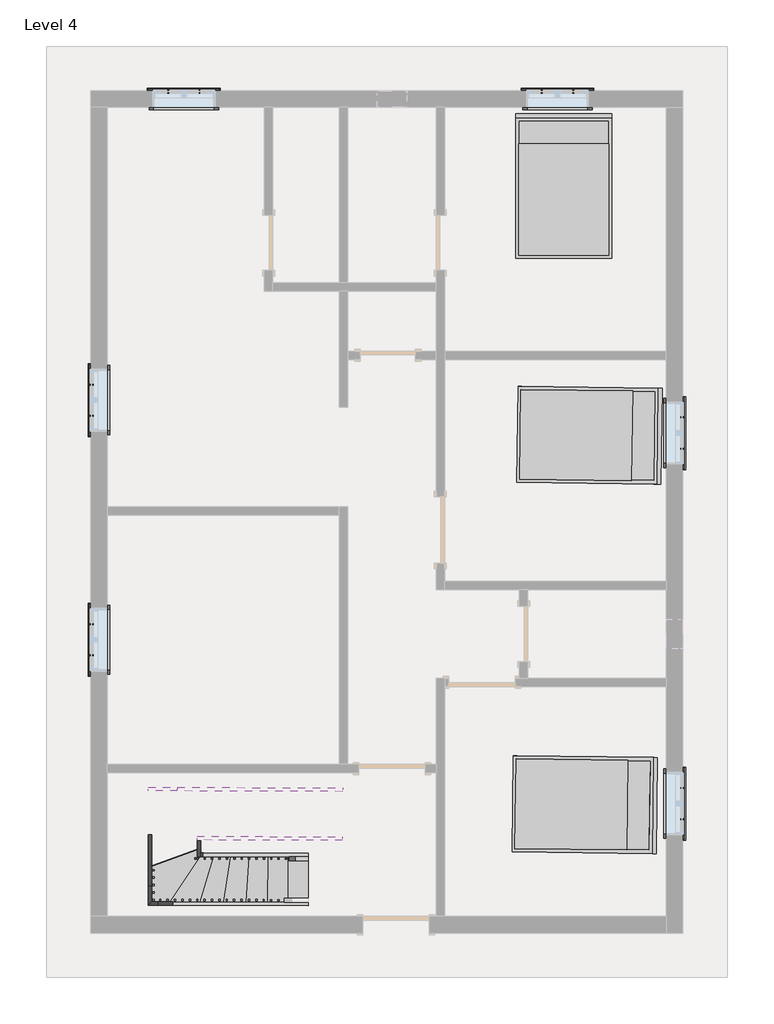
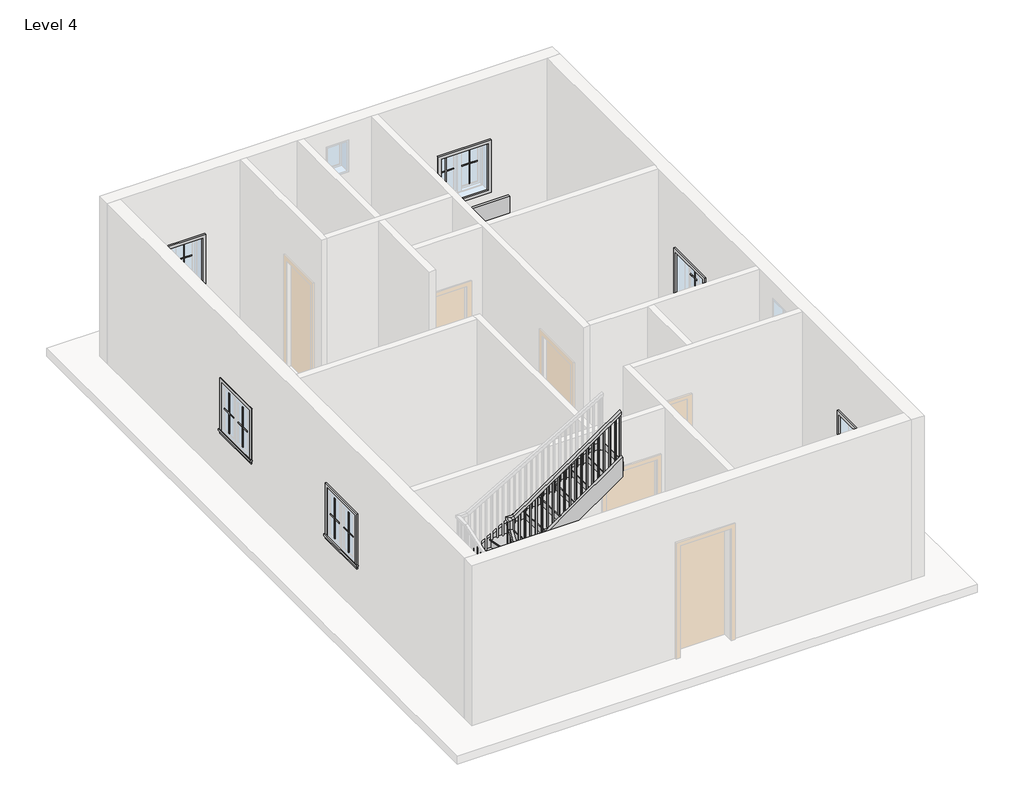
# One storey, part 3 of 3: 24 proxies, 9 members, 3 furniture elements, 1 railing, 1 stair flight.
"""IFC4 building model written with IfcOpenShell, lengths in millimetres."""

from ifc_helpers import new_model, si_unit, frame, origin, place, context, project, spatial, polyline, outline, extrude, faceted_brep, transform, mapped, element, save
from components import muntin_pattern_2x2_muntin_pattern_2x2_b3fe6957, muntin_pattern_2x2_muntin_pattern_2x2_3e0ecaf2, trim_window_exterior_flat_with_sill_41619996, trim_window_interior_flat_picture_frame_51c85655, bed_17739_bed_17739_15c61121, stair_flight_f5e35143

model = new_model("IFC4")

# Units and contexts
model_context = context("Model", 3, world=origin())
ifc_project = project(units=[si_unit("LENGTHUNIT", "METRE", prefix="MILLI")], contexts=[model_context])

# Site, building, storey
site = spatial("IfcSite", under=ifc_project)
building = spatial("IfcBuilding", under=site)
storey = spatial("IfcBuildingStorey", under=building, Name="Level 4", Elevation=6400.8)

# Proxies
placement = place(None, origin())
muntin_pattern_2x2_muntin_pattern_2x2_shape = muntin_pattern_2x2_muntin_pattern_2x2_b3fe6957(model_context)
element("IfcBuildingElementProxy", 1, Name="Muntin Pattern_2x2 : Muntin Pattern_2x2", ObjectType="Muntin Pattern_2x2 : Muntin Pattern_2x2", at=placement, inside=storey, context=model_context, shape_type="MappedRepresentation", body=[
    mapped(muntin_pattern_2x2_muntin_pattern_2x2_shape, transform((873.7257686, 6321.6571212, 7385.05), x_axis=(1.0, 0.0, 0.0), y_axis=(0.0, 1.0, 0.0), z_axis=(0.0, 0.0, 1.0))),
])
element("IfcBuildingElementProxy", 2, Name="Muntin Pattern_2x2 : Muntin Pattern_2x2", ObjectType="Muntin Pattern_2x2 : Muntin Pattern_2x2", at=placement, inside=storey, context=model_context, shape_type="MappedRepresentation", body=[
    mapped(muntin_pattern_2x2_muntin_pattern_2x2_shape, transform((2802.5382686, 1840.1446212, 7385.05), x_axis=(0.0, -1.0, 0.0), y_axis=(1.0, 0.0, 0.0), z_axis=(0.0, 0.0, 1.0))),
])
element("IfcBuildingElementProxy", 3, Name="Muntin Pattern_2x2 : Muntin Pattern_2x2", ObjectType="Muntin Pattern_2x2 : Muntin Pattern_2x2", at=placement, inside=storey, context=model_context, shape_type="MappedRepresentation", body=[
    mapped(muntin_pattern_2x2_muntin_pattern_2x2_shape, transform((2802.5382686, -3255.7303788, 7385.05), x_axis=(0.0, -1.0, 0.0), y_axis=(1.0, 0.0, 0.0), z_axis=(0.0, 0.0, 1.0))),
])
element("IfcBuildingElementProxy", 4, Name="Muntin Pattern_2x2 : Muntin Pattern_2x2", ObjectType="Muntin Pattern_2x2 : Muntin Pattern_2x2", at=placement, inside=storey, context=model_context, shape_type="MappedRepresentation", body=[
    mapped(muntin_pattern_2x2_muntin_pattern_2x2_shape, transform((-4263.4242314, 6321.6571212, 7385.05), x_axis=(1.0, 0.0, 0.0), y_axis=(0.0, 1.0, 0.0), z_axis=(0.0, 0.0, 1.0))),
])
element("IfcBuildingElementProxy", 5, Name="Muntin Pattern_2x2 : Muntin Pattern_2x2", ObjectType="Muntin Pattern_2x2 : Muntin Pattern_2x2", at=placement, inside=storey, context=model_context, shape_type="MappedRepresentation", body=[
    mapped(muntin_pattern_2x2_muntin_pattern_2x2_shape, transform((-5319.1117314, 1863.8332318, 7385.05), x_axis=(0.0, 1.0, 0.0), y_axis=(-1.0, 0.0, 0.0), z_axis=(0.0, 0.0, 1.0))),
])
element("IfcBuildingElementProxy", 6, Name="Muntin Pattern_2x2 : Muntin Pattern_2x2", ObjectType="Muntin Pattern_2x2 : Muntin Pattern_2x2", at=placement, inside=storey, context=model_context, shape_type="MappedRepresentation", body=[
    mapped(muntin_pattern_2x2_muntin_pattern_2x2_shape, transform((-5319.1117314, -1431.8167682, 7385.05), x_axis=(0.0, 1.0, 0.0), y_axis=(-1.0, 0.0, 0.0), z_axis=(0.0, 0.0, 1.0))),
])
muntin_pattern_2x2_muntin_pattern_2x2_2_shape = muntin_pattern_2x2_muntin_pattern_2x2_3e0ecaf2(model_context)
element("IfcBuildingElementProxy", 7, Name="Muntin Pattern_2x2 : Muntin Pattern_2x2", ObjectType="Muntin Pattern_2x2 : Muntin Pattern_2x2", at=placement, inside=storey, context=model_context, shape_type="MappedRepresentation", body=[
    mapped(muntin_pattern_2x2_muntin_pattern_2x2_2_shape, transform((1302.3507686, 6321.6571212, 7385.05), x_axis=(-1.0, 0.0, 0.0), y_axis=(0.0, -1.0, 0.0), z_axis=(0.0, 0.0, 1.0))),
])
element("IfcBuildingElementProxy", 8, Name="Muntin Pattern_2x2 : Muntin Pattern_2x2", ObjectType="Muntin Pattern_2x2 : Muntin Pattern_2x2", at=placement, inside=storey, context=model_context, shape_type="MappedRepresentation", body=[
    mapped(muntin_pattern_2x2_muntin_pattern_2x2_2_shape, transform((2802.5382686, 1411.5196212, 7385.05), x_axis=(0.0, 1.0, 0.0), y_axis=(-1.0, 0.0, 0.0), z_axis=(0.0, 0.0, 1.0))),
])
element("IfcBuildingElementProxy", 9, Name="Muntin Pattern_2x2 : Muntin Pattern_2x2", ObjectType="Muntin Pattern_2x2 : Muntin Pattern_2x2", at=placement, inside=storey, context=model_context, shape_type="MappedRepresentation", body=[
    mapped(muntin_pattern_2x2_muntin_pattern_2x2_2_shape, transform((2802.5382686, -3684.3553788, 7385.05), x_axis=(0.0, 1.0, 0.0), y_axis=(-1.0, 0.0, 0.0), z_axis=(0.0, 0.0, 1.0))),
])
element("IfcBuildingElementProxy", 10, Name="Muntin Pattern_2x2 : Muntin Pattern_2x2", ObjectType="Muntin Pattern_2x2 : Muntin Pattern_2x2", at=placement, inside=storey, context=model_context, shape_type="MappedRepresentation", body=[
    mapped(muntin_pattern_2x2_muntin_pattern_2x2_2_shape, transform((-3834.7992314, 6321.6571212, 7385.05), x_axis=(-1.0, 0.0, 0.0), y_axis=(0.0, -1.0, 0.0), z_axis=(0.0, 0.0, 1.0))),
])
element("IfcBuildingElementProxy", 11, Name="Muntin Pattern_2x2 : Muntin Pattern_2x2", ObjectType="Muntin Pattern_2x2 : Muntin Pattern_2x2", at=placement, inside=storey, context=model_context, shape_type="MappedRepresentation", body=[
    mapped(muntin_pattern_2x2_muntin_pattern_2x2_2_shape, transform((-5319.1117314, 2292.4582318, 7385.05), x_axis=(0.0, -1.0, 0.0), y_axis=(1.0, 0.0, 0.0), z_axis=(0.0, 0.0, 1.0))),
])
element("IfcBuildingElementProxy", 12, Name="Muntin Pattern_2x2 : Muntin Pattern_2x2", ObjectType="Muntin Pattern_2x2 : Muntin Pattern_2x2", at=placement, inside=storey, context=model_context, shape_type="MappedRepresentation", body=[
    mapped(muntin_pattern_2x2_muntin_pattern_2x2_2_shape, transform((-5319.1117314, -1003.1917682, 7385.05), x_axis=(0.0, -1.0, 0.0), y_axis=(1.0, 0.0, 0.0), z_axis=(0.0, 0.0, 1.0))),
])
trim_window_exterior_flat_with_sill_shape = trim_window_exterior_flat_with_sill_41619996(model_context)
element("IfcBuildingElementProxy", 13, Name="Trim-Window-Exterior-Flat : with Sill", ObjectType="Trim-Window-Exterior-Flat : with Sill", at=placement, inside=storey, context=model_context, shape_type="MappedRepresentation", body=[
    mapped(trim_window_exterior_flat_with_sill_shape, transform((1088.0382686, 6331.1821212, 8229.6), x_axis=(-1.0, 0.0, 0.0), y_axis=(0.0, 0.0, 1.0), z_axis=(0.0, 1.0, 0.0))),
])
element("IfcBuildingElementProxy", 14, Name="Trim-Window-Exterior-Flat : with Sill", ObjectType="Trim-Window-Exterior-Flat : with Sill", at=placement, inside=storey, context=model_context, shape_type="MappedRepresentation", body=[
    mapped(trim_window_exterior_flat_with_sill_shape, transform((2812.0632686, 1625.8321212, 8229.6), x_axis=(0.0, 1.0, 0.0), y_axis=(0.0, 0.0, 1.0), z_axis=(1.0, 0.0, 0.0))),
])
element("IfcBuildingElementProxy", 15, Name="Trim-Window-Exterior-Flat : with Sill", ObjectType="Trim-Window-Exterior-Flat : with Sill", at=placement, inside=storey, context=model_context, shape_type="MappedRepresentation", body=[
    mapped(trim_window_exterior_flat_with_sill_shape, transform((2812.0632686, -3470.0428788, 8229.6), x_axis=(0.0, 1.0, 0.0), y_axis=(0.0, 0.0, 1.0), z_axis=(1.0, 0.0, 0.0))),
])
element("IfcBuildingElementProxy", 16, Name="Trim-Window-Exterior-Flat : with Sill", ObjectType="Trim-Window-Exterior-Flat : with Sill", at=placement, inside=storey, context=model_context, shape_type="MappedRepresentation", body=[
    mapped(trim_window_exterior_flat_with_sill_shape, transform((-4049.1117314, 6331.1821212, 8229.6), x_axis=(-1.0, 0.0, 0.0), y_axis=(0.0, 0.0, 1.0), z_axis=(0.0, 1.0, 0.0))),
])
element("IfcBuildingElementProxy", 17, Name="Trim-Window-Exterior-Flat : with Sill", ObjectType="Trim-Window-Exterior-Flat : with Sill", at=placement, inside=storey, context=model_context, shape_type="MappedRepresentation", body=[
    mapped(trim_window_exterior_flat_with_sill_shape, transform((-5328.6367314, 2078.1457318, 8229.6), x_axis=(0.0, -1.0, 0.0), y_axis=(0.0, 0.0, 1.0), z_axis=(-1.0, 0.0, 0.0))),
])
element("IfcBuildingElementProxy", 18, Name="Trim-Window-Exterior-Flat : with Sill", ObjectType="Trim-Window-Exterior-Flat : with Sill", at=placement, inside=storey, context=model_context, shape_type="MappedRepresentation", body=[
    mapped(trim_window_exterior_flat_with_sill_shape, transform((-5328.6367314, -1217.5042682, 8229.6), x_axis=(0.0, -1.0, 0.0), y_axis=(0.0, 0.0, 1.0), z_axis=(-1.0, 0.0, 0.0))),
])
trim_window_interior_flat_picture_frame_shape = trim_window_interior_flat_picture_frame_51c85655(model_context)
element("IfcBuildingElementProxy", 19, Name="Trim-Window-Interior-Flat : Picture Frame", ObjectType="Trim-Window-Interior-Flat : Picture Frame", at=placement, inside=storey, context=model_context, shape_type="MappedRepresentation", body=[
    mapped(trim_window_interior_flat_picture_frame_shape, transform((1088.0382686, 6102.5821212, 8229.6), x_axis=(1.0, 0.0, 0.0), y_axis=(0.0, 0.0, 1.0), z_axis=(0.0, -1.0, 0.0))),
])
element("IfcBuildingElementProxy", 20, Name="Trim-Window-Interior-Flat : Picture Frame", ObjectType="Trim-Window-Interior-Flat : Picture Frame", at=placement, inside=storey, context=model_context, shape_type="MappedRepresentation", body=[
    mapped(trim_window_interior_flat_picture_frame_shape, transform((2583.4632686, 1625.8321212, 8229.6), x_axis=(0.0, -1.0, 0.0), y_axis=(0.0, 0.0, 1.0), z_axis=(-1.0, 0.0, 0.0))),
])
element("IfcBuildingElementProxy", 21, Name="Trim-Window-Interior-Flat : Picture Frame", ObjectType="Trim-Window-Interior-Flat : Picture Frame", at=placement, inside=storey, context=model_context, shape_type="MappedRepresentation", body=[
    mapped(trim_window_interior_flat_picture_frame_shape, transform((2583.4632686, -3470.0428788, 8229.6), x_axis=(0.0, -1.0, 0.0), y_axis=(0.0, 0.0, 1.0), z_axis=(-1.0, 0.0, 0.0))),
])
element("IfcBuildingElementProxy", 22, Name="Trim-Window-Interior-Flat : Picture Frame", ObjectType="Trim-Window-Interior-Flat : Picture Frame", at=placement, inside=storey, context=model_context, shape_type="MappedRepresentation", body=[
    mapped(trim_window_interior_flat_picture_frame_shape, transform((-4049.1117314, 6102.5821212, 8229.6), x_axis=(1.0, 0.0, 0.0), y_axis=(0.0, 0.0, 1.0), z_axis=(0.0, -1.0, 0.0))),
])
element("IfcBuildingElementProxy", 23, Name="Trim-Window-Interior-Flat : Picture Frame", ObjectType="Trim-Window-Interior-Flat : Picture Frame", at=placement, inside=storey, context=model_context, shape_type="MappedRepresentation", body=[
    mapped(trim_window_interior_flat_picture_frame_shape, transform((-5100.0367314, 2078.1457318, 8229.6), x_axis=(0.0, 1.0, 0.0), y_axis=(0.0, 0.0, 1.0), z_axis=(1.0, 0.0, 0.0))),
])
element("IfcBuildingElementProxy", 24, Name="Trim-Window-Interior-Flat : Picture Frame", ObjectType="Trim-Window-Interior-Flat : Picture Frame", at=placement, inside=storey, context=model_context, shape_type="MappedRepresentation", body=[
    mapped(trim_window_interior_flat_picture_frame_shape, transform((-5100.0367314, -1217.5042682, 8229.6), x_axis=(0.0, 1.0, 0.0), y_axis=(0.0, 0.0, 1.0), z_axis=(1.0, 0.0, 0.0))),
])

# Furniture
bed_17739_bed_17739_shape = bed_17739_bed_17739_15c61121(model_context)
element("IfcFurniture", 25, ObjectType="Bed_17739 : Bed_17739", at=placement, inside=storey, context=model_context, shape_type="MappedRepresentation", body=[
    mapped(bed_17739_bed_17739_shape, transform((1173.7632686, 4997.6821212, 6400.8), x_axis=(1.0, 0.0, 0.0), y_axis=(0.0, 1.0, 0.0), z_axis=(0.0, 0.0, 1.0))),
])
element("IfcFurniture", 26, ObjectType="Bed_17739 : Bed_17739", at=placement, inside=storey, context=model_context, shape_type="MappedRepresentation", body=[
    mapped(bed_17739_bed_17739_shape, transform((1503.3372561, 1596.4447738, 6400.8), x_axis=(-0.012740965827000846, -0.9999188306006619, 0.0), y_axis=(0.9999188306006619, -0.012740965827000846, 0.0), z_axis=(0.0, 0.0, 1.0))),
])
element("IfcFurniture", 27, ObjectType="Bed_17739 : Bed_17739", at=placement, inside=storey, context=model_context, shape_type="MappedRepresentation", body=[
    mapped(bed_17739_bed_17739_shape, transform((1438.6034215, -3483.9063624, 6400.8), x_axis=(-0.012740965827007402, -0.9999188306006618, 0.0), y_axis=(0.9999188306006618, -0.012740965827007402, 0.0), z_axis=(0.0, 0.0, 1.0))),
])

# Members
element("IfcMember", 28, ObjectType="Stringer - 2\" Width", at=placement, inside=storey, context=model_context, shape_type="SweptSolid", body=[
    extrude(outline(polyline([(-105.6436802, -202.41926), (0.0, 0.0), (2328.0658822, 0.0), (2168.9891534, -304.7999999), (90.5236019, -304.7999999), (-105.6436802, -202.41926)])), frame((-2342.1993001, -4876.8012848, 6629.1290257), z_axis=(0.003383581801438569, 0.9999942756707125, 0.0), x_axis=(-0.886519357936928, 0.002999627936996439, 0.4626817807471314)), (0.0, 0.0, 1.0), 50.8),
])
element("IfcMember", 29, ObjectType="Stringer - 2\" Width", at=placement, inside=storey, context=model_context, shape_type="SweptSolid", body=[
    extrude(outline(polyline([(-4405.9028852, -4819.0182441), (-4406.0747712, -4869.8179533), (-4542.6986856, -4869.3556725), (-4491.7270905, -4818.7278493), (-4405.9028852, -4819.0182441)])), frame((0.0, 0.0, 7362.4681426), z_axis=(0.0, 0.0, 1.0), x_axis=(1.0, 0.0, 0.0)), (0.0, 0.0, 1.0), 343.8145513),
])
element("IfcMember", 30, ObjectType="Stringer - 2\" Width", at=placement, inside=storey, context=model_context, shape_type="SweptSolid", body=[
    extrude(outline(polyline([(-4491.7270905, -4818.7278493), (-4542.6986856, -4869.3556725), (-4541.8102896, -4606.7963526), (-4491.0105804, -4606.9682386), (-4491.7270905, -4818.7278493)])), frame((0.0, 0.0, 7362.4681426), z_axis=(0.0, 0.0, 1.0), x_axis=(1.0, 0.0, 0.0)), (0.0, 0.0, 1.0), 343.8145513),
])
element("IfcMember", 31, ObjectType="Stringer - 2\" Width", at=placement, inside=storey, context=model_context, shape_type="SweptSolid", body=[
    extrude(outline(polyline([(109.7110974, -325.8403301), (0.0, 0.0), (1383.9510961, 0.0), (1489.930143, -314.7561954), (1457.0104275, -325.8403301), (109.7110974, -325.8403301)])), frame((-4491.0105804, -4606.9682386, 7362.4681426), z_axis=(-0.9999942756707125, 0.003383581801438881, 0.0), x_axis=(0.0032066921171017425, 0.9477157489074123, 0.3190996339680272)), (0.0, 0.0, 1.0), 50.8),
])
element("IfcMember", 32, ObjectType="Stringer - 2\" Width", at=placement, inside=storey, context=model_context, shape_type="SweptSolid", body=[
    extrude(outline(polyline([(-4537.3723845, -3295.2041032), (-4537.2004986, -3244.404394), (-4139.0142012, -3245.7516976), (-4139.1860871, -3296.5514068), (-4537.3723845, -3295.2041032)])), frame((0.0, 0.0, 7814.5918365), z_axis=(0.0, 0.0, 1.0), x_axis=(1.0, 0.0, 0.0)), (0.0, 0.0, 1.0), 321.6135804),
])
element("IfcMember", 33, ObjectType="Stringer - 2\" Width", at=placement, inside=storey, context=model_context, shape_type="SweptSolid", body=[
    extrude(outline(polyline([(-111.9549294, -160.635527), (0.0, 0.0), (1800.2454177, 0.0), (1587.8150598, -304.8000001), (94.8955973, -304.8), (-111.9549294, -160.635527)])), frame((-2339.9228929, -4204.0248458, 6596.6000989), z_axis=(0.003383581801438833, 0.9999942756707125, 0.0), x_axis=(-0.8204010535979692, 0.0027759099650580456, 0.5717817814334486)), (0.0, 0.0, 1.0), 50.8),
])
element("IfcMember", 34, ObjectType="Stringer - 2\" Width", at=placement, inside=storey, context=model_context, shape_type="SweptSolid", body=[
    extrude(outline(polyline([(438.5777673, -304.8), (2.5808594, -1.7936294), (3.8273846, 0.0), (400.5684618, 0.0), (819.8223258, -291.370396), (810.4891046, -304.8000001), (438.5777673, -304.8)])), frame((-3816.8461303, -4199.0275266, 7286.6862902), z_axis=(-0.9999942756707126, 0.003383581801437359, 0.0), x_axis=(0.0019309727886812906, 0.57068569595005, 0.8211663094538746)), (0.0, 0.0, 1.0), 50.8),
])
element("IfcMember", 35, ObjectType="Stringer - 2\" Width", at=placement, inside=storey, context=model_context, shape_type="SweptSolid", body=[
    extrude(outline(polyline([(213.8292849, -304.8), (0.0, 0.0), (2440.5867528, 0.0), (2654.4160377, -304.8), (213.8292849, -304.8)])), frame((-3866.8723527, -3970.2569493, 7753.8535021), z_axis=(0.003383581801438697, 0.9999942756707126, 0.0), x_axis=(0.8186346554264393, -0.0027699331781375542, 0.5743079560697587)), (0.0, 0.0, 1.0), 50.8),
])
element("IfcMember", 36, ObjectType="Stringer - 2\" Width", at=placement, inside=storey, context=model_context, shape_type="SweptSolid", body=[
    extrude(outline(polyline([(162.5062199, -277.5374274), (0.0, 0.0), (2633.4595913, 1e-07), (2795.9658112, -277.5374274), (162.5062199, -277.5374274)])), frame((-4139.1860871, -3296.5514068, 7814.5918365), z_axis=(0.0033835818014385927, 0.9999942756707125, 0.0), x_axis=(0.8629481327443969, -0.002919872311849946, 0.5052840731100094)), (0.0, 0.0, 1.0), 50.8),
])

# Railing
element("IfcRailing", 37, ObjectType="Handrail - Rectangular", at=placement, inside=storey, context=model_context, shape_type="SolidModel", body=[
    faceted_brep([(-2340.0947789, -4254.824555, 7484.5333333), (-2340.0947789, -4254.824555, 7423.1023206), (-2339.9228929, -4204.0248458, 7423.1023206), (-2339.9228929, -4204.0248458, 7484.5333333), (-3791.6181617, -4249.9131788, 8471.5092848), (-3842.4178709, -4249.7412929, 8444.6199762), (-3842.2459849, -4198.9415837, 8444.6199762), (-3791.4462757, -4199.1134696, 8471.5092848), (-1868.5796854, -3875.4177931, 10363.2), (-1868.7515713, -3926.2175023, 10363.2), (-1868.7515713, -3926.2175023, 10301.538507), (-1868.5796854, -3875.4177931, 10301.538507), (-3774.5418549, -3868.9687773, 8990.245528), (-3790.329017, -3868.9153598, 9041.045528), (-3774.7137409, -3919.7684865, 8990.245528), (-3790.500903, -3919.715069, 9041.045528), (-3791.6181617, -4249.9131788, 8687.8182666), (-3842.4178709, -4249.7412929, 8637.0182666), (-3842.2459849, -4198.9415837, 8637.0182666), (-3791.4462757, -4199.1134696, 8687.8182666), (-3918.6174347, -4249.4834639, 8687.8182666), (-3918.6174347, -4249.4834639, 8637.0182666), (-3867.6458395, -4198.8556407, 8637.0182666), (-3867.6458395, -4198.8556407, 8687.8182666), (-3918.1877198, -4122.4841909, 8687.8182666), (-3918.0978567, -4095.9257757, 8637.0182666), (-3867.2981475, -4096.0976616, 8637.0182666), (-3867.3880106, -4122.6560769, 8687.8182666), (-3917.7580049, -3995.4849179, 8870.559003), (-3917.586119, -3944.6852087, 8854.6400838), (-3866.7864097, -3944.8570947, 8854.6400838), (-3866.9582957, -3995.6568039, 8870.559003), (-3917.7580049, -3995.4849179, 9041.045528), (-3917.586119, -3944.6852087, 8990.245528), (-3866.7864097, -3944.8570947, 8990.245528), (-3866.9582957, -3995.6568039, 9041.045528), (-3917.32829, -3868.4856449, 9041.045528), (-3917.32829, -3868.4856449, 8990.245528), (-3866.7004668, -3919.4572401, 8990.245528), (-3866.7004668, -3919.4572401, 9041.045528)], [[[0, 1, 2, 3]], [[1, 0, 4, 5]], [[2, 1, 5, 6]], [[3, 2, 6, 7]], [[0, 3, 7, 4]], [[8, 9, 10, 11]], [[12, 13, 8, 11]], [[14, 12, 11, 10]], [[15, 14, 10, 9]], [[13, 15, 9, 8]], [[5, 4, 16, 17]], [[6, 5, 17, 18]], [[7, 6, 18, 19]], [[4, 7, 19, 16]], [[17, 16, 20, 21]], [[18, 17, 21, 22]], [[19, 18, 22, 23]], [[16, 19, 23, 20]], [[21, 20, 24, 25]], [[22, 21, 25, 26]], [[23, 22, 26, 27]], [[20, 23, 27, 24]], [[25, 24, 28, 29]], [[26, 25, 29, 30]], [[27, 26, 30, 31]], [[24, 27, 31, 28]], [[29, 28, 32, 33]], [[30, 29, 33, 34]], [[31, 30, 34, 35]], [[28, 31, 35, 32]], [[33, 32, 36, 37]], [[34, 33, 37, 38]], [[35, 34, 38, 39]], [[32, 35, 39, 36]], [[37, 36, 13, 12]], [[38, 37, 12, 14]], [[39, 38, 14, 15]], [[36, 39, 15, 13]]]),
    extrude(outline(polyline([(222.0468824, -19.0499999), (235.1531175, 0.0), (1186.7159363, 0.0), (1186.7159363, -19.0499999), (222.0468824, -19.0499999)])), frame((-1971.1826027, -3909.9958257, 10466.182603), z_axis=(0.0033835818014386967, 0.9999942756707125, 0.0), x_axis=(0.0, 0.0, -1.0)), (0.0, 0.0, 1.0), 19.05),
    extrude(outline(polyline([(222.0468825, -19.0499999), (235.1531175, 0.0), (1116.8160159, 0.0), (1116.8160159, -19.0499999), (222.0468825, -19.0499999)])), frame((-2072.7820211, -3909.6520537, 10396.2826826), z_axis=(0.0033835818014386967, 0.9999942756707125, 0.0), x_axis=(0.0, 0.0, -1.0)), (0.0, 0.0, 1.0), 19.05),
    extrude(outline(polyline([(222.0468825, -19.0499999), (235.1531176, 0.0), (1216.2494289, 0.0), (1216.2494289, -19.0499999), (222.0468825, -19.0499999)])), frame((-2174.3814395, -3909.3082818, 10326.3827622), z_axis=(0.0033835818014386967, 0.9999942756707125, 0.0), x_axis=(0.0, 0.0, -1.0)), (0.0, 0.0, 1.0), 19.05),
    extrude(outline(polyline([(222.0468825, -19.05), (235.1531175, 0.0), (1146.3495084, 0.0), (1146.3495084, -19.05), (222.0468825, -19.05)])), frame((-2275.980858, -3908.9645099, 10256.4828417), z_axis=(0.0033835818014386967, 0.9999942756707125, 0.0), x_axis=(0.0, 0.0, -1.0)), (0.0, 0.0, 1.0), 19.05),
    extrude(outline(polyline([(222.0468825, -19.05), (235.1531176, 0.0), (1076.449588, 0.0), (1076.449588, -19.05), (222.0468825, -19.05)])), frame((-2377.5802764, -3908.620738, 10186.5829213), z_axis=(0.0033835818014386967, 0.9999942756707125, 0.0), x_axis=(0.0, 0.0, -1.0)), (0.0, 0.0, 1.0), 19.05),
    extrude(outline(polyline([(222.0468824, -19.05), (235.1531175, 0.0), (1175.8830008, 0.0), (1175.8830008, -19.05), (222.0468824, -19.05)])), frame((-2479.1796948, -3908.2769661, 10116.6830008), z_axis=(0.0033835818014386967, 0.9999942756707125, 0.0), x_axis=(0.0, 0.0, -1.0)), (0.0, 0.0, 1.0), 19.05),
    extrude(outline(polyline([(222.0468825, -19.05), (235.1531176, 0.0), (1105.9830804, 0.0), (1105.9830804, -19.05), (222.0468825, -19.05)])), frame((-2580.7791132, -3907.9331942, 10046.7830804), z_axis=(0.0033835818014386967, 0.9999942756707125, 0.0), x_axis=(0.0, 0.0, -1.0)), (0.0, 0.0, 1.0), 19.05),
    extrude(outline(polyline([(222.0468824, -19.05), (235.1531175, 0.0), (1036.0831599, 0.0), (1036.0831599, -19.05), (222.0468824, -19.05)])), frame((-2682.3785316, -3907.5894223, 9976.8831599), z_axis=(0.0033835818014386967, 0.9999942756707125, 0.0), x_axis=(0.0, 0.0, -1.0)), (0.0, 0.0, 1.0), 19.05),
    extrude(outline(polyline([(222.0468825, -19.05), (235.1531176, 0.0), (1135.5165728, 0.0), (1135.5165728, -19.05), (222.0468825, -19.05)])), frame((-2783.97795, -3907.2456504, 9906.9832395), z_axis=(0.0033835818014386967, 0.9999942756707125, 0.0), x_axis=(0.0, 0.0, -1.0)), (0.0, 0.0, 1.0), 19.05),
    extrude(outline(polyline([(222.0468824, -19.0499999), (235.1531175, 0.0), (1065.6166523, 0.0), (1065.6166523, -19.0499999), (222.0468824, -19.0499999)])), frame((-2885.5773684, -3906.9018785, 9837.083319), z_axis=(0.0033835818014386967, 0.9999942756707125, 0.0), x_axis=(0.0, 0.0, -1.0)), (0.0, 0.0, 1.0), 19.05),
    extrude(outline(polyline([(222.0468825, -19.0499999), (235.1531176, 0.0), (995.7167319, 0.0), (995.7167319, -19.0499999), (222.0468825, -19.0499999)])), frame((-2987.1767868, -3906.5581065, 9767.1833986), z_axis=(0.0033835818014386967, 0.9999942756707125, 0.0), x_axis=(0.0, 0.0, -1.0)), (0.0, 0.0, 1.0), 19.05),
    extrude(outline(polyline([(222.0468824, -19.0499999), (235.1531175, 0.0), (1095.1501448, 0.0), (1095.1501448, -19.0499999), (222.0468824, -19.0499999)])), frame((-3088.7762052, -3906.2143346, 9697.2834781), z_axis=(0.0033835818014386967, 0.9999942756707125, 0.0), x_axis=(0.0, 0.0, -1.0)), (0.0, 0.0, 1.0), 19.05),
    extrude(outline(polyline([(222.0468825, -19.0499999), (235.1531176, 0.0), (1025.2502244, 0.0), (1025.2502244, -19.0499999), (222.0468825, -19.0499999)])), frame((-3190.3756236, -3905.8705627, 9627.3835577), z_axis=(0.0033835818014386967, 0.9999942756707125, 0.0), x_axis=(0.0, 0.0, -1.0)), (0.0, 0.0, 1.0), 19.05),
    extrude(outline(polyline([(222.0468824, -19.0499999), (235.1531175, 0.0), (1124.6836372, 0.0), (1124.6836372, -19.0499999), (222.0468824, -19.0499999)])), frame((-3291.975042, -3905.5267908, 9557.4836372), z_axis=(0.0033835818014386967, 0.9999942756707125, 0.0), x_axis=(0.0, 0.0, -1.0)), (0.0, 0.0, 1.0), 19.05),
    extrude(outline(polyline([(222.0468825, -19.0499999), (235.1531176, 0.0), (1054.7837168, 0.0), (1054.7837168, -19.0499999), (222.0468825, -19.0499999)])), frame((-3393.5744604, -3905.1830189, 9487.5837168), z_axis=(0.0033835818014386967, 0.9999942756707125, 0.0), x_axis=(0.0, 0.0, -1.0)), (0.0, 0.0, 1.0), 19.05),
    extrude(outline(polyline([(222.0468824, -19.05), (235.1531175, 0.0), (984.8837963, 0.0), (984.8837963, -19.05), (222.0468824, -19.05)])), frame((-3495.1738789, -3904.839247, 9417.6837963), z_axis=(0.0033835818014386967, 0.9999942756707125, 0.0), x_axis=(0.0, 0.0, -1.0)), (0.0, 0.0, 1.0), 19.05),
    extrude(outline(polyline([(222.0468825, -19.05), (235.1531176, 0.0), (1084.3172092, 0.0), (1084.3172092, -19.05), (222.0468825, -19.05)])), frame((-3596.7732973, -3904.4954751, 9347.7838759), z_axis=(0.0033835818014386967, 0.9999942756707125, 0.0), x_axis=(0.0, 0.0, -1.0)), (0.0, 0.0, 1.0), 19.05),
    extrude(outline(polyline([(222.0468824, -19.05), (235.1531175, 0.0), (1014.4172887, 0.0), (1014.4172887, -19.05), (222.0468824, -19.05)])), frame((-3698.3727157, -3904.1517032, 9277.8839554), z_axis=(0.0033835818014386967, 0.9999942756707125, 0.0), x_axis=(0.0, 0.0, -1.0)), (0.0, 0.0, 1.0), 19.05),
    extrude(outline(polyline([(222.0468825, -19.05), (235.1531175, 0.0), (1113.8507017, 0.0), (1113.8507017, -19.05), (222.0468825, -19.05)])), frame((-3799.9721341, -3903.8079313, 9207.984035), z_axis=(0.0033835818014386967, 0.9999942756707125, 0.0), x_axis=(0.0, 0.0, -1.0)), (0.0, 0.0, 1.0), 19.05),
    extrude(outline(polyline([(-3882.6076045, -3928.9284712), (-3901.6574955, -3928.8640139), (-3901.5930382, -3909.814123), (-3882.5431473, -3909.8785802), (-3882.6076045, -3928.9284712)])), frame((0.0, 0.0, 7924.8), z_axis=(0.0, 0.0, 1.0), x_axis=(1.0, 0.0, 0.0)), (0.0, 0.0, 1.0), 1065.445528),
    extrude(outline(polyline([(214.8944448, -19.05), (242.3055552, 0.0), (1218.1289753, 0.0), (1218.1289753, -19.05), (214.8944448, -19.05)])), frame((-3882.9513764, -4030.5278896, 8973.595642), z_axis=(-0.9999942756707125, 0.0033835818014373593, 0.0), x_axis=(0.0, 0.0, -1.0)), (0.0, 0.0, 1.0), 19.05),
    extrude(outline(polyline([(214.8944448, -19.05), (242.3055552, 0.0), (1071.9363862, 0.0), (1071.9363862, -19.05), (214.8944448, -19.05)])), frame((-3883.2951483, -4132.127308, 8827.4030529), z_axis=(-0.9999942756707125, 0.0033835818014373593, 0.0), x_axis=(0.0, 0.0, -1.0)), (0.0, 0.0, 1.0), 19.05),
    extrude(outline(polyline([(-3854.4429379, -4214.7754049), (-3854.5073951, -4233.8252959), (-3873.5572861, -4233.7608386), (-3873.4928289, -4214.7109477), (-3854.4429379, -4214.7754049)])), frame((0.0, 0.0, 7586.1333333), z_axis=(0.0, 0.0, 1.0), x_axis=(1.0, 0.0, 0.0)), (0.0, 0.0, 1.0), 1050.8849333),
    extrude(outline(polyline([(235.0765695, -19.05), (222.1234305, 0.0), (1202.0700381, 0.0), (1202.0700381, -19.05), (235.0765695, -19.05)])), frame((-3771.9578677, -4234.1046105, 8618.8700381), z_axis=(0.003383581801438833, 0.9999942756707125, 0.0), x_axis=(0.0, 0.0, -1.0)), (0.0, 0.0, 1.0), 19.05),
    extrude(outline(polyline([(235.0765695, -19.05), (222.1234305, 0.0), (1132.9866297, 0.0), (1132.9866297, -19.05), (235.0765695, -19.05)])), frame((-3670.3584493, -4234.4483825, 8549.7866297), z_axis=(0.003383581801438833, 0.9999942756707125, 0.0), x_axis=(0.0, 0.0, -1.0)), (0.0, 0.0, 1.0), 19.05),
    extrude(outline(polyline([(235.0765695, -19.05), (222.1234305, 0.0), (1233.2365546, 0.0), (1233.2365546, -19.05), (235.0765695, -19.05)])), frame((-3568.7590309, -4234.7921544, 8480.7032213), z_axis=(0.003383581801438833, 0.9999942756707125, 0.0), x_axis=(0.0, 0.0, -1.0)), (0.0, 0.0, 1.0), 19.05),
    extrude(outline(polyline([(235.0765695, -19.05), (222.1234305, 0.0), (1164.1531462, 0.0), (1164.1531462, -19.05), (235.0765695, -19.05)])), frame((-3467.1596125, -4235.1359263, 8411.6198129), z_axis=(0.003383581801438833, 0.9999942756707125, 0.0), x_axis=(0.0, 0.0, -1.0)), (0.0, 0.0, 1.0), 19.05),
    extrude(outline(polyline([(235.0765695, -19.05), (222.1234305, 0.0), (1264.4030712, 0.0), (1264.4030712, -19.05), (235.0765695, -19.05)])), frame((-3365.5601941, -4235.4796982, 8342.5364045), z_axis=(0.003383581801438833, 0.9999942756707125, 0.0), x_axis=(0.0, 0.0, -1.0)), (0.0, 0.0, 1.0), 19.05),
    extrude(outline(polyline([(235.0765695, -19.0499999), (222.1234304, 0.0), (1195.3196628, 0.0), (1195.3196628, -19.0499999), (235.0765695, -19.0499999)])), frame((-3263.9607756, -4235.8234701, 8273.4529961), z_axis=(0.003383581801438833, 0.9999942756707125, 0.0), x_axis=(0.0, 0.0, -1.0)), (0.0, 0.0, 1.0), 19.05),
    extrude(outline(polyline([(235.0765695, -19.0499999), (222.1234304, 0.0), (1295.5695877, 0.0), (1295.5695877, -19.0499999), (235.0765695, -19.0499999)])), frame((-3162.3613572, -4236.167242, 8204.3695877), z_axis=(0.003383581801438833, 0.9999942756707125, 0.0), x_axis=(0.0, 0.0, -1.0)), (0.0, 0.0, 1.0), 19.05),
    extrude(outline(polyline([(235.0765695, -19.0499999), (222.1234304, 0.0), (1226.4861793, 0.0), (1226.4861793, -19.0499999), (235.0765695, -19.0499999)])), frame((-3060.7619388, -4236.5110139, 8135.2861793), z_axis=(0.003383581801438833, 0.9999942756707125, 0.0), x_axis=(0.0, 0.0, -1.0)), (0.0, 0.0, 1.0), 19.05),
    extrude(outline(polyline([(235.0765695, -19.0499999), (222.1234304, 0.0), (1157.4027709, 0.0), (1157.4027709, -19.0499999), (235.0765695, -19.0499999)])), frame((-2959.1625204, -4236.8547858, 8066.2027709), z_axis=(0.003383581801438833, 0.9999942756707125, 0.0), x_axis=(0.0, 0.0, -1.0)), (0.0, 0.0, 1.0), 19.05),
    extrude(outline(polyline([(235.0765695, -19.0499999), (222.1234304, 0.0), (1257.6526958, 0.0), (1257.6526958, -19.0499999), (235.0765695, -19.0499999)])), frame((-2857.563102, -4237.1985577, 7997.1193625), z_axis=(0.003383581801438833, 0.9999942756707125, 0.0), x_axis=(0.0, 0.0, -1.0)), (0.0, 0.0, 1.0), 19.05),
    extrude(outline(polyline([(235.0765695, -19.0499999), (222.1234304, 0.0), (1188.5692874, 0.0), (1188.5692874, -19.0499999), (235.0765695, -19.0499999)])), frame((-2755.9636836, -4237.5423297, 7928.0359541), z_axis=(0.003383581801438833, 0.9999942756707125, 0.0), x_axis=(0.0, 0.0, -1.0)), (0.0, 0.0, 1.0), 19.05),
    extrude(outline(polyline([(235.0765696, -19.05), (222.1234305, 0.0), (1119.4858791, 0.0), (1119.4858791, -19.05), (235.0765696, -19.05)])), frame((-2654.3642652, -4237.8861016, 7858.9525458), z_axis=(0.003383581801438833, 0.9999942756707125, 0.0), x_axis=(0.0, 0.0, -1.0)), (0.0, 0.0, 1.0), 19.05),
    extrude(outline(polyline([(235.0765696, -19.05), (222.1234305, 0.0), (1219.7358041, 0.0), (1219.7358041, -19.05), (235.0765696, -19.05)])), frame((-2552.7648468, -4238.2298735, 7789.8691374), z_axis=(0.003383581801438833, 0.9999942756707125, 0.0), x_axis=(0.0, 0.0, -1.0)), (0.0, 0.0, 1.0), 19.05),
    extrude(outline(polyline([(235.0765696, -19.05), (222.1234305, 0.0), (1150.6523957, 0.0), (1150.6523957, -19.05), (235.0765696, -19.05)])), frame((-2451.1654284, -4238.5736454, 7720.785729), z_axis=(0.003383581801438833, 0.9999942756707125, 0.0), x_axis=(0.0, 0.0, -1.0)), (0.0, 0.0, 1.0), 19.05),
    extrude(outline(polyline([(-3882.5216615, -3903.5286166), (-3901.5715525, -3903.4641593), (-3901.5070953, -3884.4142684), (-3882.4572043, -3884.4787256), (-3882.5216615, -3903.5286166)])), frame((0.0, 0.0, 7924.8), z_axis=(0.0, 0.0, 1.0), x_axis=(1.0, 0.0, 0.0)), (0.0, 0.0, 1.0), 1065.445528),
    extrude(outline(polyline([(-3883.574463, -4214.6768355), (-3883.6389202, -4233.7267264), (-3902.6888112, -4233.6622692), (-3902.624354, -4214.6123782), (-3883.574463, -4214.6768355)])), frame((0.0, 0.0, 7586.1333333), z_axis=(0.0, 0.0, 1.0), x_axis=(1.0, 0.0, 0.0)), (0.0, 0.0, 1.0), 1050.8849333),
    extrude(outline(polyline([(222.0468825, -19.0499999), (235.1531176, 0.0), (1244.1187228, 0.0), (1244.1187228, -19.0499999), (222.0468825, -19.0499999)])), frame((-1887.7477479, -3910.2781359, 10523.5853895), z_axis=(0.0033835818014386967, 0.9999942756707125, 0.0), x_axis=(0.0, 0.0, -1.0)), (0.0, 0.0, 1.0), 19.05),
    extrude(outline(polyline([(235.0765695, -19.05), (222.1234305, 0.0), (1088.0455568, 0.0), (1088.0455568, -19.05), (235.0765695, -19.05)])), frame((-2359.0909555, -4238.8851887, 7658.1788901), z_axis=(0.003383581801438833, 0.9999942756707125, 0.0), x_axis=(0.0, 0.0, -1.0)), (0.0, 0.0, 1.0), 19.05),
])

# Stair flight
stair_flight_shape = stair_flight_f5e35143(model_context)
element("IfcStairFlight", 38, ObjectType="2\" Tread 1\" Nosing 1/4\" Riser", at=placement, inside=storey, context=model_context, shape_type="MappedRepresentation", body=[
    mapped(stair_flight_shape, transform((0.0, 0.0, 0.0), x_axis=(1.0, 0.0, 0.0), y_axis=(0.0, 1.0, 0.0), z_axis=(0.0, 0.0, 1.0))),
])

save(model, "model.ifc")

# Revit data of these elements
# Type "Muntin Pattern_2x2 : Muntin Pattern_2x2"
#   Width [instance default] = 4' - 0"
#   Thickness = 0' - 0 1/2"
#   Height [instance default] = 4' - 0"
#   Distance = 0' - 0 3/4"
#   Interior Material [instance default] = none
#   Exterior Material [instance default] = none
#   Default Elevation = 0
# Type "Trim-Window-Exterior-Flat : with Sill"
#   Trim Width = 0' - 2 1/4"
#   Trim Thickness_Picture Frame = 0' - 1 1/4"
#   Trim Thickness_with Sill = 0' - 0 3/4"
#   Sill Thickness = 0' - 1 1/4"
#   Opening Width [instance default] = 2' - 0"
#   Opening Height [instance default] = 3' - 0"
#   Default Elevation = 4' - 0"
#   Sill = yes
#   Picture Frame = no
#   Trim Material [instance default] = none
# Type "Trim-Window-Interior-Flat : Picture Frame"
#   Trim Thickness_Picture Frame = 0' - 1 1/4"
#   Trim Width = 0' - 2 1/4"
#   Trim Thickness_with Sill = 0' - 0 3/4"
#   Sill Thickness = 0' - 1 1/4"
#   Opening Width [instance default] = 2' - 0"
#   Opening Height [instance default] = 3' - 0"
#   Default Elevation = 4' - 0"
#   Sill = no
#   Picture Frame = yes
#   Trim Material [instance default] = none
# Type "Bed_17739 : Bed_17739"
#   Default Elevation = 0
# Type "Handrail - Rectangular"
#   Assembly Code = "C2010400"
#   built-in parameter 1008612 = 0.0416667 (stored number, unit not read)
#   built-in parameter 1008611 = 0.0416667 (stored number, unit not read)
#   built-in parameter 1008609 = 0.333333 (stored number, unit not read)
#   built-in parameter 1008604 = 0.166667 (stored number, unit not read)
#   built-in parameter 1008603 = 0.166667 (stored number, unit not read)
#   Railing Height = 3' - 0"
#   built-in parameter 1008630 = 2
#   built-in parameter 1008610 = 2
#   built-in parameter 1008618 = Baluster - Square : 3/4"
# Elements 1, 2, 3, 4, 5, 6, 7, 8, 9, 10, 11, 12 (IfcBuildingElementProxy, "Muntin Pattern_2x2 : Muntin Pattern_2x2")
#   Width = 0' - 11 5/8"
#   Height = 2' - 6 1/2"
#   Interior Material = Wood - Stained
#   Exterior Material = Clad - White
#   Phase Created = New Construction
#   Materials on its faces: "Clad - White", "Wood - Stained"
# Elements 13, 14, 15, 16, 17, 18 (IfcBuildingElementProxy, "Trim-Window-Exterior-Flat : with Sill")
#   Opening Width = 2' - 10"
#   Opening Height = 3' - 0"
#   Trim Material = Clad - White
#   Phase Created = New Construction
#   Materials on its faces: "Clad - White"
# Elements 19, 20, 21, 22, 23, 24 (IfcBuildingElementProxy, "Trim-Window-Interior-Flat : Picture Frame")
#   Opening Width = 2' - 10"
#   Opening Height = 3' - 0"
#   Trim Material = Wood - Stained
#   Phase Created = New Construction
#   Materials on its faces: "Wood - Stained"
# Elements 25, 26, 27 (IfcFurniture, "Bed_17739 : Bed_17739")
#   Phase Created = New Construction
#   Materials on its faces: "legs", "sheets", "bed frame", "Blanket"
# Elements 28, 29, 30, 31, 32, 33, 34, 35, 36 (IfcMember, "Stringer - 2\" Width")
#   Phase Created = New Construction
# Element 37 (IfcRailing, "Handrail - Rectangular")
#   Phase Created = New Construction
# Element 38 (IfcStairFlight, "2\" Tread 1\" Nosing 1/4\" Riser")
#   Phase Created = New Construction
# Materials
#   "Clad - White": class "Wood", colour RGB 242 242 238, transparency 0, Cost = 0
#   "Wood - Stained": class "Wood", colour RGB 224 178 126, transparency 0, Cost = 0
#   "legs": colour RGB 90 73 37, transparency 0, Cost = 0
#   "sheets": colour RGB 200 195 176, transparency 0, Cost = 0
#   "bed frame": colour RGB 90 73 37, transparency 0, Cost = 0
#   "Blanket": class "System", colour RGB 59 0 1, transparency 0, Cost = 0
